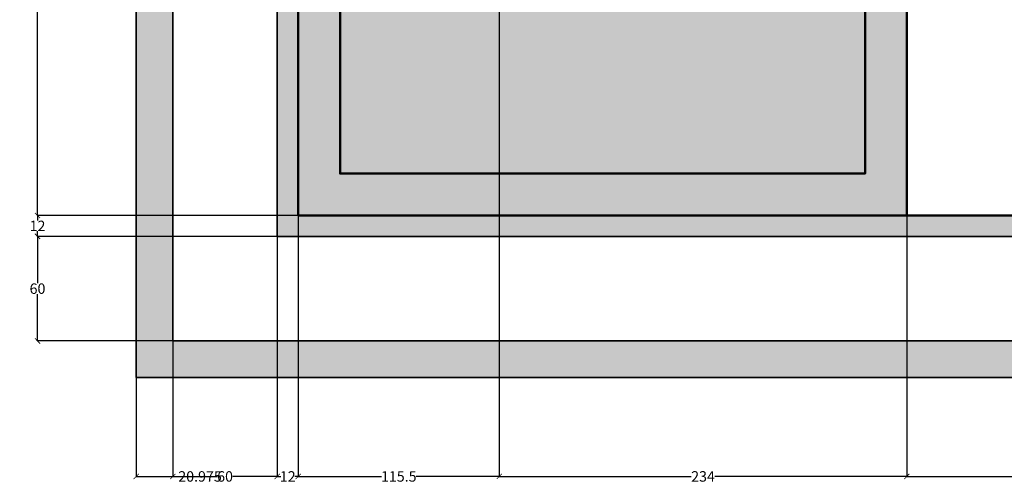
# Model space of a CAD drawing. Units: inches. Extents: x 925 to 2834, y 111 to 1355.
# Tile 1 of 25: x 925 to 1490, y 111 to 377. Entities that reach past the tile are written whole.
import ezdxf

# ---------------------------------------------------------------- set-up
doc = ezdxf.new("R2010")
doc.units = ezdxf.units.IN
doc.header["$MEASUREMENT"] = 0
for name, color, linetype, lineweight in [('A-ANNO-DIMS', 2, 'Continuous', 18), ('A-ANNO-TTLB', 7, 'Continuous', 35), ('A-FLOR-PATT', 252, 'Continuous', 13), ('A-WALL', 7, 'Continuous', 50)]:
    doc.layers.add(name, color=color, linetype=linetype, lineweight=lineweight)
doc.styles.get("Standard").update_dxf_attribs({"font": 'arial.ttf'})
doc.dimstyles.get("Standard").update_dxf_attribs({"dimtxt": 6, "dimasz": 3, "dimexe": 0.18, "dimexo": 0.0625, "dimgap": 0.09, "dimtad": 0, "dimtih": 1, "dimtoh": 1, "dimdec": 1, "dimzin": 0, "dimdsep": 46, "dimlunit": 3, "dimtxsty": 'Standard', "dimblk": 'ARCHTICK', "dimcen": 0.09, "dimadec": 0, "dimazin": 0, "dimtfac": 1, "dimtdec": 1, "dimtofl": 0, "dimtmove": 0, "dimatfit": 3, "dimfxl": 1, "dimtolj": 1, "dimtzin": 0, "dimarcsym": 0})

# ---------------------------------------------------------------- blocks, each defined once
blk = doc.blocks.new('_ArchTick')
at = {"color": 0, "linetype": 'ByBlock', "const_width": 0.15}
blk.add_lwpolyline([(-0.5, -0.5), (0.5, 0.5)], dxfattribs=at)
blk = doc.blocks.new('*D22')
at = {"layer": 'A-ANNO-DIMS', "color": 0, "lineweight": -2, "transparency": 16777216}
for p, q in [((1012.71, 193.03), (1012.71, 115.18)), ((991.74, 172.05), (991.74, 115.18)), ((991.74, 115.36), (1012.71, 115.36)), ((1012.71, 115.36), (1015.71, 115.36))]:
    blk.add_line(p, q, dxfattribs=at)
at = {"layer": 'Defpoints', "color": 0, "transparency": 16777216}
for p in [(1012.71, 193.09), (991.74, 172.11), (1012.71, 115.36)]:
    blk.add_point(p, dxfattribs=at)
at = {"layer": 'A-ANNO-DIMS', "color": 0, "lineweight": -2, "transparency": 16777216, "xscale": 3, "yscale": 3, "zscale": 3, "rotation": 180}
blk.add_blockref('_ArchTick', (991.74, 115.36), dxfattribs=at)
at = {"layer": 'A-ANNO-DIMS', "color": 0, "lineweight": -2, "transparency": 16777216, "xscale": 3, "yscale": 3, "zscale": 3}
blk.add_blockref('_ArchTick', (1012.71, 115.36), dxfattribs=at)
at = {"layer": 'A-ANNO-DIMS', "color": 0, "transparency": 16777216, "insert": (1028.33, 115.36), "char_height": 6, "attachment_point": 5}
blk.add_mtext('\\A1;20.975', dxfattribs=at)
blk = doc.blocks.new('*D23')
at = {"layer": 'A-ANNO-DIMS', "color": 0, "lineweight": -2, "transparency": 16777216}
for p, q in [((1072.71, 253.03), (1072.71, 115.18)), ((1012.71, 193.03), (1012.71, 115.18)), ((1012.71, 115.36), (1038.32, 115.36)), ((1072.71, 115.36), (1047.11, 115.36))]:
    blk.add_line(p, q, dxfattribs=at)
at = {"layer": 'Defpoints', "color": 0, "transparency": 16777216}
for p in [(1072.71, 253.09), (1012.71, 193.09), (1072.71, 115.36)]:
    blk.add_point(p, dxfattribs=at)
at = {"layer": 'A-ANNO-DIMS', "color": 0, "lineweight": -2, "transparency": 16777216, "xscale": 3, "yscale": 3, "zscale": 3, "rotation": 180}
blk.add_blockref('_ArchTick', (1012.71, 115.36), dxfattribs=at)
at = {"layer": 'A-ANNO-DIMS', "color": 0, "lineweight": -2, "transparency": 16777216, "xscale": 3, "yscale": 3, "zscale": 3}
blk.add_blockref('_ArchTick', (1072.71, 115.36), dxfattribs=at)
at = {"layer": 'A-ANNO-DIMS', "color": 0, "transparency": 16777216, "insert": (1042.71, 115.36), "char_height": 6, "attachment_point": 5}
blk.add_mtext('\\A1;60', dxfattribs=at)
blk = doc.blocks.new('*D24')
at = {"layer": 'A-ANNO-DIMS', "color": 0, "lineweight": -2, "transparency": 16777216}
for p, q in [((1084.71, 265.03), (1084.71, 115.18)), ((1072.71, 253.03), (1072.71, 115.18)), ((1072.71, 115.36), (1074.64, 115.36)), ((1084.71, 115.36), (1082.79, 115.36))]:
    blk.add_line(p, q, dxfattribs=at)
at = {"layer": 'Defpoints', "color": 0, "transparency": 16777216}
for p in [(1084.71, 265.09), (1072.71, 253.09), (1084.71, 115.36)]:
    blk.add_point(p, dxfattribs=at)
at = {"layer": 'A-ANNO-DIMS', "color": 0, "lineweight": -2, "transparency": 16777216, "xscale": 3, "yscale": 3, "zscale": 3, "rotation": 180}
blk.add_blockref('_ArchTick', (1072.71, 115.36), dxfattribs=at)
at = {"layer": 'A-ANNO-DIMS', "color": 0, "lineweight": -2, "transparency": 16777216, "xscale": 3, "yscale": 3, "zscale": 3}
blk.add_blockref('_ArchTick', (1084.71, 115.36), dxfattribs=at)
at = {"layer": 'A-ANNO-DIMS', "color": 0, "transparency": 16777216, "insert": (1078.71, 115.36), "char_height": 6, "attachment_point": 5}
blk.add_mtext('\\A1;12', dxfattribs=at)
blk = doc.blocks.new('*D25')
at = {"layer": 'A-ANNO-DIMS', "color": 0, "lineweight": -2, "transparency": 16777216}
for p, q in [((1200.21, 727.53), (1200.21, 115.18)), ((1084.71, 265.03), (1084.71, 115.18)), ((1084.71, 115.36), (1132.51, 115.36)), ((1200.21, 115.36), (1152.42, 115.36))]:
    blk.add_line(p, q, dxfattribs=at)
at = {"layer": 'Defpoints', "color": 0, "transparency": 16777216}
for p in [(1200.21, 727.59), (1084.71, 265.09), (1200.21, 115.36)]:
    blk.add_point(p, dxfattribs=at)
at = {"layer": 'A-ANNO-DIMS', "color": 0, "lineweight": -2, "transparency": 16777216, "xscale": 3, "yscale": 3, "zscale": 3, "rotation": 180}
blk.add_blockref('_ArchTick', (1084.71, 115.36), dxfattribs=at)
at = {"layer": 'A-ANNO-DIMS', "color": 0, "lineweight": -2, "transparency": 16777216, "xscale": 3, "yscale": 3, "zscale": 3}
blk.add_blockref('_ArchTick', (1200.21, 115.36), dxfattribs=at)
at = {"layer": 'A-ANNO-DIMS', "color": 0, "transparency": 16777216, "insert": (1142.46, 115.36), "char_height": 6, "attachment_point": 5}
blk.add_mtext('\\A1;115.5', dxfattribs=at)
blk = doc.blocks.new('*D26')
at = {"layer": 'A-ANNO-DIMS', "color": 0, "lineweight": -2, "transparency": 16777216}
for p, q in [((1200.21, 727.53), (1200.21, 115.18)), ((1434.21, 385.03), (1434.21, 115.18)), ((1200.21, 115.36), (1310.46, 115.36)), ((1434.21, 115.36), (1323.97, 115.36))]:
    blk.add_line(p, q, dxfattribs=at)
at = {"layer": 'Defpoints', "color": 0, "transparency": 16777216}
for p in [(1200.21, 727.59), (1434.21, 385.09), (1434.21, 115.36)]:
    blk.add_point(p, dxfattribs=at)
at = {"layer": 'A-ANNO-DIMS', "color": 0, "lineweight": -2, "transparency": 16777216, "xscale": 3, "yscale": 3, "zscale": 3, "rotation": 180}
blk.add_blockref('_ArchTick', (1200.21, 115.36), dxfattribs=at)
at = {"layer": 'A-ANNO-DIMS', "color": 0, "lineweight": -2, "transparency": 16777216, "xscale": 3, "yscale": 3, "zscale": 3}
blk.add_blockref('_ArchTick', (1434.21, 115.36), dxfattribs=at)
at = {"layer": 'A-ANNO-DIMS', "color": 0, "transparency": 16777216, "insert": (1317.21, 115.36), "char_height": 6, "attachment_point": 5}
blk.add_mtext('\\A1;234', dxfattribs=at)
blk = doc.blocks.new('*D27')
at = {"layer": 'A-ANNO-DIMS', "color": 0, "lineweight": -2, "transparency": 16777216}
for p, q in [((1621.21, 395.03), (1621.21, 115.18)), ((1434.21, 385.03), (1434.21, 115.18)), ((1434.21, 115.36), (1521.28, 115.36)), ((1621.21, 115.36), (1534.15, 115.36))]:
    blk.add_line(p, q, dxfattribs=at)
at = {"layer": 'Defpoints', "color": 0, "transparency": 16777216}
for p in [(1621.21, 395.09), (1434.21, 385.09), (1621.21, 115.36)]:
    blk.add_point(p, dxfattribs=at)
at = {"layer": 'A-ANNO-DIMS', "color": 0, "lineweight": -2, "transparency": 16777216, "xscale": 3, "yscale": 3, "zscale": 3, "rotation": 180}
blk.add_blockref('_ArchTick', (1434.21, 115.36), dxfattribs=at)
at = {"layer": 'A-ANNO-DIMS', "color": 0, "lineweight": -2, "transparency": 16777216, "xscale": 3, "yscale": 3, "zscale": 3}
blk.add_blockref('_ArchTick', (1621.21, 115.36), dxfattribs=at)
at = {"layer": 'A-ANNO-DIMS', "color": 0, "transparency": 16777216, "insert": (1527.71, 115.36), "char_height": 6, "attachment_point": 5}
blk.add_mtext('\\A1;187', dxfattribs=at)
blk = doc.blocks.new('*D32')
at = {"layer": 'A-ANNO-DIMS', "color": 0, "lineweight": -2, "transparency": 16777216}
for p, q in [((1072.65, 253.09), (934.81, 253.09)), ((934.99, 253.09), (934.99, 226.24)), ((934.99, 193.09), (934.99, 219.94)), ((1012.65, 193.09), (934.81, 193.09))]:
    blk.add_line(p, q, dxfattribs=at)
at = {"layer": 'Defpoints', "color": 0, "transparency": 16777216}
for p in [(934.99, 253.09), (1072.71, 253.09), (1012.71, 193.09)]:
    blk.add_point(p, dxfattribs=at)
at = {"layer": 'A-ANNO-DIMS', "color": 0, "lineweight": -2, "transparency": 16777216, "xscale": 3, "yscale": 3, "zscale": 3}
for p, rotation in [((934.99, 253.09), 90), ((934.99, 193.09), 270)]:
    blk.add_blockref('_ArchTick', p, dxfattribs=dict(at, rotation=rotation))
at = {"layer": 'A-ANNO-DIMS', "color": 0, "transparency": 16777216, "insert": (934.99, 223.09), "char_height": 6, "attachment_point": 5}
blk.add_mtext('\\A1;60', dxfattribs=at)
blk = doc.blocks.new('*D33')
at = {"layer": 'A-ANNO-DIMS', "color": 0, "lineweight": -2, "transparency": 16777216}
for p, q in [((1084.65, 265.09), (934.81, 265.09)), ((934.99, 265.09), (934.99, 262.19)), ((934.99, 253.09), (934.99, 255.99)), ((1072.65, 253.09), (934.81, 253.09))]:
    blk.add_line(p, q, dxfattribs=at)
at = {"layer": 'Defpoints', "color": 0, "transparency": 16777216}
for p in [(934.99, 265.09), (1084.71, 265.09), (1072.71, 253.09)]:
    blk.add_point(p, dxfattribs=at)
at = {"layer": 'A-ANNO-DIMS', "color": 0, "lineweight": -2, "transparency": 16777216, "xscale": 3, "yscale": 3, "zscale": 3}
for p, rotation in [((934.99, 265.09), 90), ((934.99, 253.09), 270)]:
    blk.add_blockref('_ArchTick', p, dxfattribs=dict(at, rotation=rotation))
at = {"layer": 'A-ANNO-DIMS', "color": 0, "transparency": 16777216, "insert": (934.99, 259.09), "char_height": 6, "attachment_point": 5}
blk.add_mtext('\\A1;12', dxfattribs=at)
blk = doc.blocks.new('*D34')
at = {"layer": 'A-ANNO-DIMS', "color": 0, "lineweight": -2, "transparency": 16777216}
for p, q in [((1084.65, 530.59), (934.81, 530.59)), ((934.99, 530.59), (934.99, 400.99)), ((934.99, 265.09), (934.99, 394.69)), ((1084.65, 265.09), (934.81, 265.09))]:
    blk.add_line(p, q, dxfattribs=at)
at = {"layer": 'Defpoints', "color": 0, "transparency": 16777216}
for p in [(934.99, 530.59), (1084.71, 530.59), (1084.71, 265.09)]:
    blk.add_point(p, dxfattribs=at)
at = {"layer": 'A-ANNO-DIMS', "color": 0, "lineweight": -2, "transparency": 16777216, "xscale": 3, "yscale": 3, "zscale": 3}
for p, rotation in [((934.99, 530.59), 90), ((934.99, 265.09), 270)]:
    blk.add_blockref('_ArchTick', p, dxfattribs=dict(at, rotation=rotation))
at = {"layer": 'A-ANNO-DIMS', "color": 0, "transparency": 16777216, "insert": (934.99, 397.84), "char_height": 6, "attachment_point": 5}
blk.add_mtext('\\A1;265.5', dxfattribs=at)

msp = doc.modelspace()

# ---------------------------------------------------------------- hatches: boundary and pattern name
at = {"layer": 'A-FLOR-PATT', "transparency": 33554605}
h = msp.add_hatch(color=256, dxfattribs=at)
h.dxf.hatch_style = 1
h.paths.add_polyline_path([(1931.688, 1294.5638), (991.7375, 1294.5638), (991.7375, 172.1134), (1931.688, 172.1134)])
h.paths.add_polyline_path([(1910.7128, 1273.5886), (1910.7128, 193.0886), (1012.7128, 193.0886), (1012.7128, 1273.5886)], flags=16)
h.paths.add_polyline_path([(1850.7128, 1213.5886), (1850.7128, 253.0886), (1072.7128, 253.0886), (1072.7128, 1213.5886)], flags=0)
h.paths.add_polyline_path([(1838.7128, 1201.5886), (1838.7128, 265.0886), (1084.7128, 265.0886), (1084.7128, 530.5886), (1084.7128, 1201.5886)], flags=0)
h.paths.add_polyline_path([(1547.6758, 1155.7396), (1547.6758, 1119.115), (1513.0687, 1119.115), (1513.0687, 1155.7396)], flags=0)
h.paths.add_polyline_path([(1600.1067, 1154.9439), (1634.7139, 1154.9439), (1634.7139, 1119.115), (1600.1067, 1119.115)], flags=0)
h.paths.add_polyline_path([(1505.2502, 1144.5358), (1505.2502, 1119.115), (1470.643, 1119.115), (1470.643, 1144.5358)], flags=0)
h.paths.add_polyline_path([(1559.1357, 1141.0962), (1593.7428, 1141.0962), (1593.7428, 1119.115), (1559.1357, 1119.115)], flags=0)
h.paths.add_polyline_path([(1462.8966, 1154.9439), (1462.8966, 1119.115), (1428.2895, 1119.115), (1428.2895, 1154.9439)], flags=0)
h.paths.add_polyline_path([(1642.4603, 1144.5358), (1677.0675, 1144.5358), (1677.0675, 1119.115), (1642.4603, 1119.115)], flags=0)
h.paths.add_polyline_path([(1422.3508, 1141.0962), (1422.3508, 1119.115), (1387.7436, 1119.115), (1387.7436, 1141.0962)], flags=0)
h.paths.add_polyline_path([(1684.8859, 1155.7396), (1719.4931, 1155.7396), (1719.4931, 1119.115), (1684.8859, 1119.115)], flags=0)
h.paths.add_polyline_path([(1718.7128, 1081.5886), (1718.7128, 1050.1249), (1715.7128, 1050.1249), (1715.7128, 1026.1249), (1715.7128, 1002.1249), (1718.7128, 1002.1249), (1730.7128, 1002.1249), (1730.7128, 998.1249), (1730.7128, 990.1249), (1730.7128, 986.1249), (1718.7128, 986.1249), (1718.7128, 893.5886), (1715.3735, 893.5886), (1715.3735, 891.5886), (1713.3735, 891.5886, 0.41421356), (1677.3735, 855.5886), (1713.3735, 855.5886), (1713.3735, 853.5886), (1715.3735, 853.5886), (1715.3735, 851.5886), (1718.7128, 851.5886), (1718.7128, 821.5865), (1734.4655, 821.5865), (1734.3735, 819.5886, -0.41421356), (1712.4415, 793.5886), (1712.4415, 791.5886), (1718.7128, 791.5886), (1718.7128, 717.5886), (1718.7128, 669.5886), (1732.7128, 669.5886), (1732.7128, 665.5886), (1732.7128, 641.5886), (1732.7128, 634.5886), (1732.7128, 610.5886), (1732.7128, 603.5886), (1718.7128, 603.5886), (1718.7128, 385.0886), (1434.2128, 385.0886), (1434.2128, 530.5886), (1410.2128, 530.5886), (1408.2128, 530.5886), (1408.2128, 532.5886, 0.41421356), (1372.2128, 568.5886), (1372.2128, 532.5886), (1370.2128, 532.5886), (1370.2128, 530.5886), (1368.2128, 530.5886), (1282.2128, 530.5886), (1210.2128, 530.5886), (1200.2128, 530.5886), (1200.2128, 542.1915), (1183.2307, 542.1915), (1183.2307, 546.1915), (1200.2128, 546.1915), (1200.2128, 572.1915), (1183.2307, 572.1915), (1183.2307, 576.1915), (1200.2128, 576.1915), (1200.2128, 727.5886), (1210.2128, 727.5886), (1234.2128, 727.5886), (1259.7128, 727.5886), (1259.7128, 775.5886), (1259.7128, 799.5886), (1259.7128, 847.5886), (1259.7128, 993.5872), (1259.7128, 1065.5872), (1259.7128, 1071.5886), (1219.6318, 1071.5886), (1219.6318, 1081.5886), (1084.7128, 1081.5886), (1084.7128, 1119.115), (1256.8974, 1119.115), (1256.8974, 1154.9439), (1291.5046, 1154.9439), (1291.5046, 1119.115), (1256.8974, 1119.115), (1256.6723, 1081.5886), (1293.7128, 1081.5886), (1341.7128, 1081.5886), (1341.7128, 1093.5886), (1347.7128, 1093.5886), (1371.7128, 1093.5886), (1377.7128, 1093.5886), (1377.7128, 1081.5886), (1668.7128, 1081.5886), (1668.7128, 1117.5886), (1675.7128, 1117.5886), (1711.7128, 1117.5886), (1718.7128, 1117.5886)], flags=0)
h.paths.add_polyline_path([(1376.2838, 1155.7396), (1376.2838, 1119.115), (1341.6766, 1119.115), (1341.6766, 1155.7396)], flags=0)
h.paths.add_polyline_path([(1341.7128, 1076.0886), (1293.7128, 1076.0886), (1293.7128, 1071.5886), (1269.7128, 1071.5886), (1269.7128, 1065.5872), (1266.7128, 1065.5872), (1266.7128, 1029.5872), (1265.7128, 1029.5872), (1265.7128, 993.5872), (1269.7128, 993.5872), (1269.7128, 903.5886), (1269.7128, 893.5886), (1269.7128, 847.5886), (1265.2128, 847.5886), (1265.2128, 799.5886), (1269.7128, 799.5886), (1269.7128, 775.5886), (1265.2128, 775.5886), (1265.2128, 727.5886), (1269.7128, 727.5886), (1444.2128, 727.5886), (1444.2128, 717.5886), (1234.2128, 717.5886), (1234.2128, 722.0886), (1210.2128, 722.0886), (1210.2128, 717.5886), (1210.2128, 540.5886), (1210.2128, 536.0886), (1282.2128, 536.0886), (1282.2128, 535.0886), (1210.2128, 535.0886), (1210.2128, 540.5886), (1210.2128, 717.5886), (1210.2128, 723.0886), (1234.2128, 723.0886), (1234.2128, 717.5886), (1444.2128, 717.5886), (1444.2128, 727.5886), (1269.7128, 727.5886), (1264.2128, 727.5886), (1264.2128, 775.5886), (1269.7128, 775.5886), (1269.7128, 799.5886), (1264.2128, 799.5886), (1264.2128, 847.5886), (1269.7128, 847.5886), (1269.7128, 893.5886), (1269.7128, 903.5886), (1269.7128, 993.5872), (1264.7128, 993.5872), (1264.7128, 1029.5872), (1265.7128, 1029.5872), (1265.7128, 1065.5872), (1269.7128, 1065.5872), (1269.7128, 1071.5886), (1293.7128, 1071.5886), (1293.7128, 1077.0886), (1341.7128, 1077.0886)], flags=0)
h.paths.add_polyline_path([(1730.9529, 1141.0962), (1765.5601, 1141.0962), (1765.5601, 1119.115), (1730.9529, 1119.115)], flags=0)
h.paths.add_polyline_path([(1333.8582, 1144.5358), (1333.8582, 1119.115), (1299.251, 1119.115), (1299.251, 1144.5358)], flags=0)
h.paths.add_polyline_path([(1592.7128, 968.5886), (1596.0342, 968.5886), (1602.7128, 968.5886), (1708.7128, 968.5886), (1708.7128, 903.5886), (1602.7128, 903.5886), (1602.7128, 938.5886), (1592.7128, 938.5886), (1592.7128, 903.5886), (1451.7128, 903.5886), (1451.7128, 893.5886), (1511.7128, 893.5886), (1511.7128, 881.5886), (1515.2128, 881.5886), (1518.7128, 881.5886), (1518.7128, 893.5886), (1592.7128, 893.5886), (1592.7128, 799.5886), (1518.7128, 799.5886), (1518.7128, 857.5886), (1511.7128, 857.5886), (1511.7128, 799.5886), (1511.7128, 772.0886), (1521.7128, 772.0886), (1521.7128, 792.5886), (1592.7128, 792.5886), (1592.7128, 727.5886), (1521.7128, 727.5886), (1521.7128, 748.0886), (1511.7128, 748.0886), (1511.7128, 717.5886), (1708.7128, 717.5886), (1714.2128, 717.5886), (1714.2128, 669.5886), (1708.7128, 669.5886), (1708.7128, 641.5886), (1492.2128, 641.5886), (1492.2128, 631.5886), (1621.2128, 631.5886), (1621.2128, 443.0886), (1625.7128, 443.0886), (1625.7128, 503.0886), (1625.7128, 507.5886), (1625.7128, 631.5886), (1708.7128, 631.5886), (1708.7128, 507.5886), (1655.7128, 507.5886), (1655.7128, 503.0886), (1708.7128, 503.0886), (1708.7128, 395.0886), (1625.7128, 395.0886), (1625.7128, 419.0886), (1621.2128, 419.0886), (1621.2128, 395.0886), (1482.2128, 395.0886), (1482.2128, 385.0886), (1434.2128, 385.0886), (1434.2128, 433.0886), (1444.2128, 433.0886), (1444.2128, 631.5886), (1450.2128, 631.5886), (1450.2128, 634.91), (1452.2128, 634.91), (1452.2128, 669.5886), (1454.2128, 669.5886, -0.40021217), (1490.1712, 635.3173), (1492.2128, 635.3173), (1492.2128, 641.5886), (1564.7128, 641.5886), (1564.7128, 677.5886), (1672.7128, 677.5886), (1672.7128, 681.5886), (1564.7128, 681.5886), (1564.7128, 717.5886), (1511.7128, 717.5886), (1511.7128, 748.0886), (1511.7128, 772.0886), (1511.7128, 799.5886), (1511.7128, 857.5886), (1511.8913, 857.5886), (1511.8913, 859.5886), (1515.6201, 859.5886, 0.41421356), (1537.552, 879.5886), (1513.552, 879.5886), (1511.8913, 879.5886), (1511.8913, 881.5886), (1511.7128, 881.5886), (1511.7128, 893.5886), (1451.7128, 893.5886), (1451.7128, 903.5886), (1592.7128, 903.5886), (1592.7128, 938.5886), (1592.7128, 940.5886), (1596.4415, 940.5886, 0.41421356), (1618.3735, 966.5886), (1594.3735, 966.5886), (1592.7128, 966.5886)], flags=0)
h.paths.add_polyline_path([(1377.7128, 903.5886), (1377.7128, 893.5886), (1305.7128, 893.5886), (1305.7128, 903.5886)], flags=0)
h.paths.add_polyline_path([(1708.7128, 821.5886), (1712.0342, 821.5886), (1712.0342, 819.5886), (1710.3735, 819.5886), (1708.7128, 819.5886)], flags=0)
h.paths.add_polyline_path([(1576.7128, 695.1992), (1575.5896, 693.6649), (1575.9687, 694.6994), (1575.4438, 695.1992), (1575.9687, 695.699), (1575.5896, 696.7335)], flags=0)
h.paths.add_polyline_path([(1565.9817, 662.3134), (1565.4568, 661.8136), (1565.8359, 660.7791), (1564.7128, 662.3134), (1565.8359, 663.8477), (1565.4568, 662.8132)], flags=0)
h.paths.add_polyline_path([(1444.2128, 433.0886), (1444.2128, 395.0886), (1482.2128, 395.0886), (1482.2128, 389.0886), (1438.2128, 389.0886), (1438.2128, 391.8608), (1438.2128, 433.0886)], flags=0)
h.paths.add_polyline_path([(1410.2128, 506.5886), (1410.2128, 289.0886), (1108.7128, 289.0886), (1108.7128, 506.5886)], flags=0)
h.paths.add_polyline_path([(1612.3153, 838.3016), (1680.4151, 838.3016), (1680.4151, 851.3131), (1612.3153, 851.3131)], flags=8)
h.paths.add_polyline_path([(1208.3174, 395.0436), (1282.1017, 395.0436), (1282.1017, 408.0552), (1208.3174, 408.0552)], flags=8)
h.paths.add_polyline_path([(1291.8049, 598.7427), (1369.8017, 598.7427), (1369.8017, 611.7542), (1291.8049, 611.7542)], flags=8)
h.paths.add_polyline_path([(1119.679, 917.3022), (1191.0817, 917.3022), (1191.0817, 930.3137), (1119.679, 930.3137)], flags=8)
h.paths.add_polyline_path([(1332.2261, 815.9808), (1410.2258, 815.9808), (1410.2258, 829.001), (1332.2261, 829.001)], flags=8)
h.paths.add_polyline_path([(1390.9013, 955.8158), (1475.4981, 955.8158), (1475.4981, 968.8273), (1390.9013, 968.8273)], flags=8)
h.paths.add_polyline_path([(1620.3436, 998.9325), (1688.4434, 998.9325), (1688.4434, 1011.944), (1620.3436, 1011.944)], flags=8)
h.paths.add_polyline_path([(1620.3436, 914.1039), (1691.7405, 914.1039), (1691.7405, 927.1155), (1620.3436, 927.1155)], flags=8)
h.paths.add_polyline_path([(1521.4542, 816.005), (1589.5569, 816.005), (1589.5569, 829.0253), (1521.4542, 829.0253)], flags=8)
h.paths.add_polyline_path([(1528.524, 740.3497), (1602.3082, 740.3497), (1602.3082, 753.3613), (1528.524, 753.3613)], flags=8)
h.paths.add_polyline_path([(1627.6094, 762.6128), (1702.3091, 762.6128), (1702.3091, 775.6244), (1627.6094, 775.6244)], flags=8)
h.paths.add_polyline_path([(1610.5442, 657.2751), (1684.3284, 657.2751), (1684.3284, 670.2867), (1610.5442, 670.2867)], flags=8)
h.paths.add_polyline_path([(1636.6983, 519.472), (1711.3981, 519.472), (1711.3981, 532.4835), (1636.6983, 532.4835)], flags=8)
h.paths.add_polyline_path([(1616.8577, 424.8539), (1694.8545, 424.8539), (1694.8545, 437.8654), (1616.8577, 437.8654)], flags=8)
h.paths.add_polyline_path([(1506.1456, 460.8838), (1579.9299, 460.8838), (1579.9299, 473.8953), (1506.1456, 473.8953)], flags=8)
h.paths.add_polyline_path([(1624.6119, 784.6011), (1696.9185, 784.6011), (1696.9185, 797.7864), (1624.6119, 797.7864)], flags=8)
h.paths.add_polyline_path([(1606.3732, 854.2194), (1683.3039, 854.2194), (1683.3039, 867.4048), (1606.3732, 867.4048)], flags=8)
h.paths.add_polyline_path([(1127.8008, 940.3581), (1165.1637, 940.3581), (1165.1637, 953.5348), (1127.8008, 953.5348)], flags=8)
h.paths.add_polyline_path([(1620.8657, 1019.4968), (1677.3447, 1019.4968), (1677.3447, 1032.6735), (1620.8657, 1032.6735)], flags=8)
h.paths.add_polyline_path([(1620.8643, 930.1821), (1703.0564, 930.1821), (1703.0564, 943.3675), (1620.8643, 943.3675)], flags=8)
h.paths.add_polyline_path([(1324.5702, 836.8338), (1408.0892, 836.8338), (1408.0892, 850.0191), (1324.5702, 850.0191)], flags=8)
h.paths.add_polyline_path([(1281.6584, 622.8885), (1383.6213, 622.8885), (1383.6213, 636.0739), (1281.6584, 636.0739)], flags=8)
h.paths.add_polyline_path([(1210.6721, 416.7893), (1269.1299, 416.7893), (1269.1299, 429.9747), (1210.6721, 429.9747)], flags=8)
h.paths.add_polyline_path([(1507.8264, 477.4836), (1586.7329, 477.4836), (1586.7329, 490.669), (1507.8264, 490.669)], flags=8)
h.paths.add_polyline_path([(1643.6238, 443.8135), (1696.6696, 443.8135), (1696.6696, 456.5643), (1643.6238, 456.5643)], flags=8)
h.paths.add_polyline_path([(1647.2466, 540.5638), (1693.1825, 540.5638), (1693.1825, 553.7491), (1647.2466, 553.7491)], flags=8)
h.paths.add_polyline_path([(1626.0633, 668.5064), (1673.3174, 668.5064), (1673.3174, 681.6831), (1626.0633, 681.6831)], flags=8)
h.paths.add_polyline_path([(1538.2915, 830.7872), (1567.5942, 830.7872), (1567.5942, 843.5293), (1538.2915, 843.5293)], flags=8)
h.paths.add_polyline_path([(1530.9338, 754.0477), (1559.576, 754.0477), (1559.576, 766.7898), (1530.9338, 766.7898)], flags=8)
h.paths.add_polyline_path([(1351.2461, 979.2309), (1513.8919, 979.2309), (1513.8919, 992.4076), (1351.2461, 992.4076)], flags=8)
at = {"layer": 'A-FLOR-PATT'}
h = msp.add_hatch(color=256, dxfattribs=at)
h.dxf.hatch_style = 1
h.paths.add_polyline_path([(1850.7128, 1213.5886), (1072.7128, 1213.5886), (1072.7128, 253.0886), (1850.7128, 253.0886)])
h.paths.add_polyline_path([(1084.7128, 1201.5886), (1838.7128, 1201.5886), (1838.7128, 265.0886), (1084.7128, 265.0886)], flags=16)
h.paths.add_polyline_path([(1183.2307, 576.1915), (1200.2128, 576.1915), (1200.2128, 727.5886), (1210.2128, 727.5886), (1234.2128, 727.5886), (1259.7128, 727.5886), (1259.7128, 775.5886), (1259.7128, 799.5886), (1259.7128, 847.5886), (1259.7128, 993.5872), (1259.7128, 1065.5872), (1259.7128, 1071.5886), (1219.6318, 1071.5886), (1219.6318, 1081.5886), (1293.7128, 1081.5886), (1341.7128, 1081.5886), (1341.7128, 1093.5886), (1347.7128, 1093.5886), (1347.7128, 1081.5886), (1371.7128, 1081.5886), (1371.7128, 1093.5886), (1377.7128, 1093.5886), (1377.7128, 1081.5886), (1668.7128, 1081.5886), (1668.7128, 1117.5886), (1675.7128, 1117.5886), (1675.7128, 1081.5886), (1711.7128, 1081.5886), (1711.7128, 1117.5886), (1718.7128, 1117.5886), (1718.7128, 1081.5886), (1718.7128, 1050.1249), (1715.7128, 1050.1249), (1715.7128, 1026.1249), (1715.7128, 1002.1249), (1718.7128, 1002.1249), (1730.7128, 1002.1249), (1730.7128, 998.1249), (1730.7128, 990.1249), (1730.7128, 986.1249), (1718.7128, 986.1249), (1718.7128, 893.5886), (1715.3735, 893.5886), (1715.3735, 891.5886), (1713.3735, 891.5886, 0.41421356), (1677.3735, 855.5886), (1713.3735, 855.5886), (1713.3735, 853.5886), (1715.3735, 853.5886), (1715.3735, 851.5886), (1718.7128, 851.5886), (1718.7128, 821.5865), (1734.4655, 821.5865), (1734.3735, 819.5886, -0.41421356), (1712.4415, 793.5886), (1712.4415, 791.5886), (1718.7128, 791.5886), (1718.7128, 717.5886), (1718.7128, 669.5886), (1732.7128, 669.5886), (1732.7128, 665.5886), (1732.7128, 641.5886), (1732.7128, 634.5886), (1732.7128, 610.5886), (1732.7128, 603.5886), (1718.7128, 603.5886), (1718.7128, 385.0886), (1434.2128, 385.0886), (1434.2128, 433.0886), (1434.2128, 530.5886), (1410.2128, 530.5886), (1408.2128, 530.5886), (1408.2128, 532.5886, 0.41421356), (1372.2128, 568.5886), (1372.2128, 532.5886), (1370.2128, 532.5886), (1370.2128, 530.5886), (1368.2128, 530.5886), (1282.2128, 530.5886), (1210.2128, 530.5886), (1200.2128, 530.5886), (1200.2128, 542.1915), (1183.2307, 542.1915), (1183.2307, 546.1915), (1200.2128, 546.1915), (1200.2128, 572.1915), (1183.2307, 572.1915)], flags=0)
h.paths.add_polyline_path([(1210.2128, 717.5886), (1210.2128, 723.0886), (1234.2128, 723.0886), (1234.2128, 717.5886), (1444.2128, 717.5886), (1444.2128, 727.5886), (1269.7128, 727.5886), (1264.2128, 727.5886), (1264.2128, 775.5886), (1269.7128, 775.5886), (1269.7128, 799.5886), (1264.2128, 799.5886), (1264.2128, 847.5886), (1269.7128, 847.5886), (1269.7128, 893.5886), (1269.7128, 903.5886), (1269.7128, 993.5872), (1264.7128, 993.5872), (1264.7128, 1029.5872), (1265.7128, 1029.5872), (1265.7128, 1065.5872), (1269.7128, 1065.5872), (1269.7128, 1071.5886), (1293.7128, 1071.5886), (1293.7128, 1077.0886), (1341.7128, 1077.0886), (1341.7128, 1076.0886), (1293.7128, 1076.0886), (1293.7128, 1071.5886), (1269.7128, 1071.5886), (1269.7128, 1065.5872), (1266.7128, 1065.5872), (1266.7128, 1029.5872), (1265.7128, 1029.5872), (1265.7128, 993.5872), (1269.7128, 993.5872), (1269.7128, 903.5886), (1269.7128, 893.5886), (1269.7128, 847.5886), (1265.2128, 847.5886), (1265.2128, 799.5886), (1269.7128, 799.5886), (1269.7128, 775.5886), (1265.2128, 775.5886), (1265.2128, 727.5886), (1269.7128, 727.5886), (1444.2128, 727.5886), (1444.2128, 717.5886), (1234.2128, 717.5886), (1234.2128, 722.0886), (1210.2128, 722.0886), (1210.2128, 717.5886), (1210.2128, 540.5886), (1210.2128, 536.0886), (1282.2128, 536.0886), (1282.2128, 535.0886), (1210.2128, 535.0886), (1210.2128, 540.5886)], flags=0)
h.paths.add_polyline_path([(1450.2128, 634.91), (1452.2128, 634.91), (1452.2128, 669.5886), (1454.2128, 669.5886, -0.40021217), (1490.1712, 635.3173), (1492.2128, 635.3173), (1492.2128, 641.5886), (1564.7128, 641.5886), (1564.7128, 677.5886), (1672.7128, 677.5886), (1672.7128, 681.5886), (1564.7128, 681.5886), (1564.7128, 717.5886), (1511.7128, 717.5886), (1511.7128, 748.0886), (1511.7128, 772.0886), (1511.7128, 799.5886), (1511.7128, 857.5886), (1511.8913, 857.5886), (1511.8913, 859.5886), (1515.6201, 859.5886, 0.41421356), (1537.552, 879.5886), (1513.552, 879.5886), (1511.8913, 879.5886), (1511.8913, 881.5886), (1511.7128, 881.5886), (1511.7128, 893.5886), (1451.7128, 893.5886), (1451.7128, 903.5886), (1592.7128, 903.5886), (1592.7128, 938.5886), (1592.7128, 940.5886), (1596.4415, 940.5886, 0.41421356), (1618.3735, 966.5886), (1594.3735, 966.5886), (1592.7128, 966.5886), (1592.7128, 968.5886), (1596.0342, 968.5886), (1602.7128, 968.5886), (1708.7128, 968.5886), (1708.7128, 903.5886), (1602.7128, 903.5886), (1602.7128, 938.5886), (1592.7128, 938.5886), (1592.7128, 903.5886), (1451.7128, 903.5886), (1451.7128, 893.5886), (1511.7128, 893.5886), (1511.7128, 881.5886), (1518.7128, 881.5886), (1518.7128, 893.5886), (1592.7128, 893.5886), (1592.7128, 799.5886), (1518.7128, 799.5886), (1518.7128, 857.5886), (1511.7128, 857.5886), (1511.7128, 799.5886), (1511.7128, 772.0886), (1521.7128, 772.0886), (1521.7128, 792.5886), (1592.7128, 792.5886), (1592.7128, 727.5886), (1521.7128, 727.5886), (1521.7128, 748.0886), (1511.7128, 748.0886), (1511.7128, 717.5886), (1708.7128, 717.5886), (1714.2128, 717.5886), (1714.2128, 669.5886), (1708.7128, 669.5886), (1708.7128, 641.5886), (1492.2128, 641.5886), (1492.2128, 631.5886), (1621.2128, 631.5886), (1621.2128, 443.0886), (1625.7128, 443.0886), (1625.7128, 503.0886), (1625.7128, 507.5886), (1625.7128, 631.5886), (1708.7128, 631.5886), (1708.7128, 507.5886), (1655.7128, 507.5886), (1655.7128, 503.0886), (1708.7128, 503.0886), (1708.7128, 395.0886), (1625.7128, 395.0886), (1625.7128, 419.0886), (1621.2128, 419.0886), (1621.2128, 395.0886), (1482.2128, 395.0886), (1482.2128, 389.0886), (1438.2128, 389.0886), (1438.2128, 391.8608), (1438.2128, 433.0886), (1444.2128, 433.0886), (1444.2128, 631.5886), (1450.2128, 631.5886)], flags=0)
h.paths.add_polyline_path([(1444.2128, 433.0886), (1444.2128, 395.0886), (1482.2128, 395.0886), (1482.2128, 391.0886), (1440.2128, 391.0886), (1440.2128, 391.8608), (1440.2128, 433.0886)], flags=0)
h.paths.add_polyline_path([(1305.7128, 893.5886), (1305.7128, 903.5886), (1377.7128, 903.5886), (1377.7128, 893.5886)], flags=0)
h.paths.add_polyline_path([(1564.7128, 662.3134), (1565.8359, 663.8477), (1565.4568, 662.8132), (1565.9817, 662.3134), (1565.4568, 661.8136), (1565.8359, 660.7791)], flags=0)
h.paths.add_polyline_path([(1575.4438, 695.1992), (1575.9687, 695.699), (1575.5896, 696.7335), (1576.7128, 695.1992), (1575.5896, 693.6649), (1575.9687, 694.6994)], flags=0)
h.paths.add_polyline_path([(1708.7128, 821.5886), (1712.0342, 821.5886), (1712.0342, 819.5886), (1710.3735, 819.5886), (1708.7128, 819.5886)], flags=0)
at = {"layer": 'A-FLOR-PATT', "transparency": 33554498}
h = msp.add_hatch(color=256, dxfattribs=at)
h.dxf.hatch_style = 1
h.paths.add_polyline_path([(1434.2128, 530.5886), (1084.7128, 530.5886), (1084.7128, 265.0886), (1434.2128, 265.0886)])
h.paths.add_polyline_path([(1410.2128, 506.5886), (1410.2128, 289.0886), (1108.7128, 289.0886), (1108.7128, 506.5886)], flags=16)
h.paths.add_polyline_path([(1410.2128, 506.5886), (1108.7128, 506.5886), (1108.7128, 289.0886), (1410.2128, 289.0886)], flags=16)

# ---------------------------------------------------------------- linework, layer by layer
at = {"layer": 'A-ANNO-TTLB'}
msp.add_line((1838.7128, 265.0886), (1084.7128, 265.0886), dxfattribs=at)
for points in [[(991.7375, 172.1134), (1931.688, 172.1134), (1931.688, 1294.5638), (991.7375, 1294.5638)], [(1012.7128, 193.0886), (1910.7128, 193.0886), (1910.7128, 1273.5886), (1012.7128, 1273.5886)], [(1072.7128, 253.0886), (1850.7128, 253.0886), (1850.7128, 1213.5886), (1072.7128, 1213.5886)], [(1084.7128, 265.0886), (1838.7128, 265.0886), (1838.7128, 1201.5886), (1084.7128, 1201.5886)]]:
    msp.add_lwpolyline(points, close=True, dxfattribs=at)
at = {"layer": 'A-WALL'}
for p, q in [((1084.7128, 530.5886), (1084.7128, 265.0886)), ((1434.2128, 385.0886), (1434.2128, 265.0886)), ((1434.2128, 265.0886), (1434.2128, 385.0886)), ((1084.7128, 265.0886), (1460.2128, 265.0886)), ((1434.2128, 265.0886), (1838.7128, 265.0886))]:
    msp.add_line(p, q, dxfattribs=at)
for points in [[(1434.2128, 530.5886), (1084.7128, 530.5886), (1084.7128, 265.0886), (1434.2128, 265.0886)], [(1410.2128, 506.5886), (1108.7128, 506.5886), (1108.7128, 289.0886), (1410.2128, 289.0886)]]:
    msp.add_lwpolyline(points, close=True, dxfattribs=at)

# ---------------------------------------------------------------- dimensions: what is measured, and where the dimension line sits
at = {"layer": 'A-ANNO-DIMS'}
for base, p1, p2, override, picture, middle in [((1200.2128, 115.3634), (1084.7128, 265.0886), (1200.2128, 727.5886), {"dimdec": 1, "dimlfac": 1, "dimrnd": 0, "dimzin": 0, "dimdsep": 46, "dimlunit": 2}, '*D25', (1142.4628, 115.3634)), ((1434.2128, 115.3634), (1200.2128, 727.5886), (1434.2128, 385.0886), {"dimdec": 0, "dimlfac": 1, "dimrnd": 0, "dimzin": 0, "dimdsep": 46, "dimlunit": 2}, '*D26', (1317.2128, 115.3634)), ((1621.2128, 115.3634), (1434.2128, 385.0886), (1621.2128, 395.0886), {"dimdec": 0, "dimlfac": 1, "dimrnd": 0, "dimzin": 0, "dimdsep": 46, "dimlunit": 2}, '*D27', (1527.7128, 115.3634)), ((1084.7128, 115.3634), (1072.7128, 253.0886), (1084.7128, 265.0886), {"dimdec": 0, "dimlfac": 1, "dimrnd": 0, "dimzin": 0, "dimdsep": 46, "dimlunit": 2}, '*D24', (1078.7128, 115.3634)), ((1072.7128, 115.3634), (1012.7128, 193.0886), (1072.7128, 253.0886), {"dimdec": 0, "dimlfac": 1, "dimrnd": 0, "dimzin": 0, "dimdsep": 46, "dimlunit": 2}, '*D23', (1042.7128, 115.3634)), ((1012.7128, 115.3634), (991.7375, 172.1134), (1012.7128, 193.0886), {"dimdec": 3, "dimlfac": 1, "dimrnd": 0, "dimzin": 0, "dimdsep": 46, "dimlunit": 2}, '*D22', (1028.3307, 115.3634))]:
    dim = msp.add_linear_dim(base=base, p1=p1, p2=p2, dimstyle='Standard', override=override, dxfattribs=at)
    dim.commit()
    dim.dimension.update_dxf_attribs({"geometry": picture, "text_midpoint": middle})
for base, p1, p2, override, picture, middle in [((934.9875, 530.5886), (1084.7128, 265.0886), (1084.7128, 530.5886), {"dimdec": 1, "dimlfac": 1, "dimrnd": 0, "dimzin": 0, "dimdsep": 46, "dimlunit": 2}, '*D34', (934.9875, 397.8386)), ((934.9875, 265.0886), (1072.7128, 253.0886), (1084.7128, 265.0886), {"dimdec": 0, "dimlfac": 1, "dimrnd": 0, "dimzin": 0, "dimdsep": 46, "dimlunit": 2}, '*D33', (934.9875, 259.0886)), ((934.9875, 253.0886), (1012.7128, 193.0886), (1072.7128, 253.0886), {"dimdec": 0, "dimlfac": 1, "dimrnd": 0, "dimzin": 0, "dimdsep": 46, "dimlunit": 2}, '*D32', (934.9875, 223.0886))]:
    dim = msp.add_linear_dim(base=base, p1=p1, p2=p2, angle=90, dimstyle='Standard', override=override, dxfattribs=at)
    dim.commit()
    dim.dimension.update_dxf_attribs({"geometry": picture, "text_midpoint": middle})

doc.saveas('drawing.dxf')
